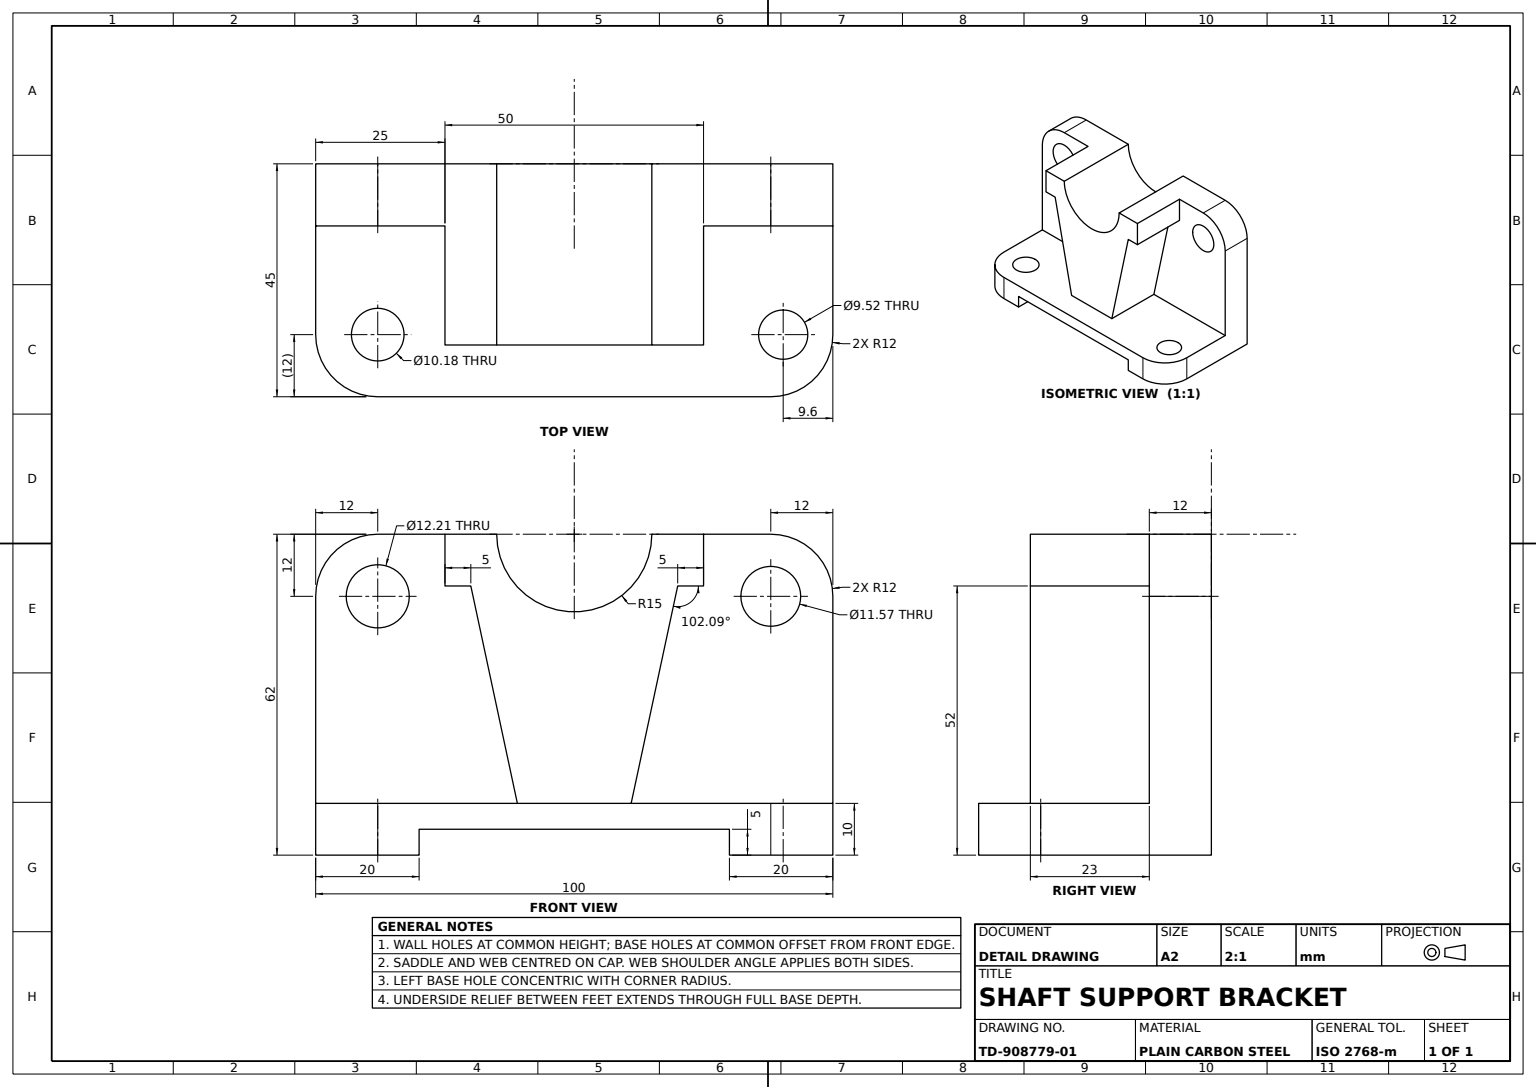
SolidWorks part; units mm, degrees
material "Plain Carbon Steel"
ref_plane "Front Plane" through (0, 0, 0) normal (0, 0, 1) x (1, 0, 0)
ref_plane "Top Plane" through (0, 0, 0) normal (0, 1, 0) x (1, 0, 0)
ref_plane "Right Plane" through (0, 0, 0) normal (1, 0, 0) x (0, 0, -1)
sketch "Base Plate Profile" plane through (0, 0, 0) normal (0, 0, 1) x (1, 0, 0)
  line L0 (0, 0) -> (20, 0)
  line L1 (20, 0) -> (20, 5)
  line L2 (20, 5) -> (80, 5)
  line L3 (80, 5) -> (80, 0)
  line L4 (80, 0) -> (100, 0)
  line L5 (100, 0) -> (100, 10)
  line L6 (100, 10) -> (0, 10)
  line L7 (0, 10) -> (0, 0)
  dimension "D1" = 20
  dimension "D2" = 20
  dimension "D3" = 100
  dimension "D4" = 10
  dimension "D5" = 80
  dimension "D6" = 5
extrude "Base Plate" add sketch "Base Plate Profile" along normal mid plane 45 contours L6 L7 L0 L1 L2 L3 L4 L5
sketch "Back Wall Sketch" plane through (100, 0, 0) normal (1, 0, 0) x (0, 0, -1)
  line L0 (22.5, 10) -> (10.5, 10)
  line L1 (-22.5, 10) -> (22.5, 10) construction
  line L2 (10.5, 10) -> (10.5, 62)
  line L3 (10.5, 62) -> (22.5, 62)
  line L4 (22.5, 62) -> (22.5, 10)
  dimension "D1" = 12
  dimension "D2" = 52
extrude "Back Wall" add sketch "Back Wall Sketch" against normal blind 100 contours L2 L3 L4 L0
sketch "Saddle Support Profile" plane through (0, 0, -10.5) normal (0, 0, 1) x (1, 0, 0)
  line L0 (39, 10) -> (61, 10)
  line L1 (0, 10) -> (100, 10) construction
  line L2 (100, 10) -> (0, 10) construction
  line L5 (75, 52) -> (75, 62)
  line L6 (0, 62) -> (100, 62) construction
  line L7 (75, 62) -> (65, 62)
  line L8 (25, 62) -> (25, 52)
  line L11 (25, 52) -> (30, 52)
  line L12 (30, 52) -> (39, 10)
  line L13 (50, 5) -> (50, 75.4057) construction
  line L14 (20, 5) -> (80, 5) construction
  line L15 (75, 52) -> (70, 52)
  line L16 (70, 52) -> (61, 10)
  line L17 (35, 62) -> (25, 62)
  arc A0 (35, 62) -> (65, 62) centre (50, 62) ccw
  dimension "D11" = 15
  dimension "D1" = 50
  dimension "D2" = 5
  dimension "D3" = 11
  dimension "D4" = 10
  dimension "D5" = 10
  dimension "D6" = 25
  dimension "D7" = 22
  dimension "D8" = 5
  dimension "D9" = 30
extrude "Saddle Support" add sketch "Saddle Support Profile" along normal blind 23
sketch "Wall Holes Sketch" plane through (0, 0, -10.5) normal (0, 0, 1) x (1, 0, 0)
  line L0 (35, 62) -> (65, 62) construction
  line L1 (0, 10) -> (0, 62) construction
  line L2 (0, 62) -> (25, 62) construction
  line L3 (75, 62) -> (100, 62) construction
  line L6 (100, 10) -> (100, 62) construction
  circle A0 centre (50, 62) radius 15
  circle A1 centre (12, 50) radius 6.1025
  circle A2 centre (88, 50) radius 5.7831
  dimension "D5" = 12.205
  dimension "D6" = 11.5662
  dimension "D7" = 30
  dimension "D1" = 12
  dimension "D2" = 12
  dimension "D3" = 12
  dimension "D4" = 12
extrude "Wall Holes" cut sketch "Wall Holes Sketch" against normal through all
fillet "Wall Corner Fillets R12" radius 12 4 edges at (0, 5, 22.5) (100, 62, -16.5) (0, 62, -16.5) (100, 5, 22.5)
sketch "Base Mounting Holes Sketch" plane through (0, 10, 0) normal (0, 1, 0) x (1, 0, 0)
  line L0 (0, -10.5) -> (0, 10.5) construction
  line L1 (88, -22.5) -> (12, -22.5) construction
  line L2 (100, -10.5) -> (100, 10.5) construction
  circle A0 centre (12, -10.5) radius 5.0906
  circle A1 centre (90.3965, -10.5) radius 4.7622
  dimension "D5" = 10.1812
  dimension "D6" = 9.5244
  dimension "D1" = 12
  dimension "D2" = 12
  dimension "D3" = 9.6035
  dimension "D4" = 12
extrude "Base Mounting Holes" cut sketch "Base Mounting Holes Sketch" against normal through all
